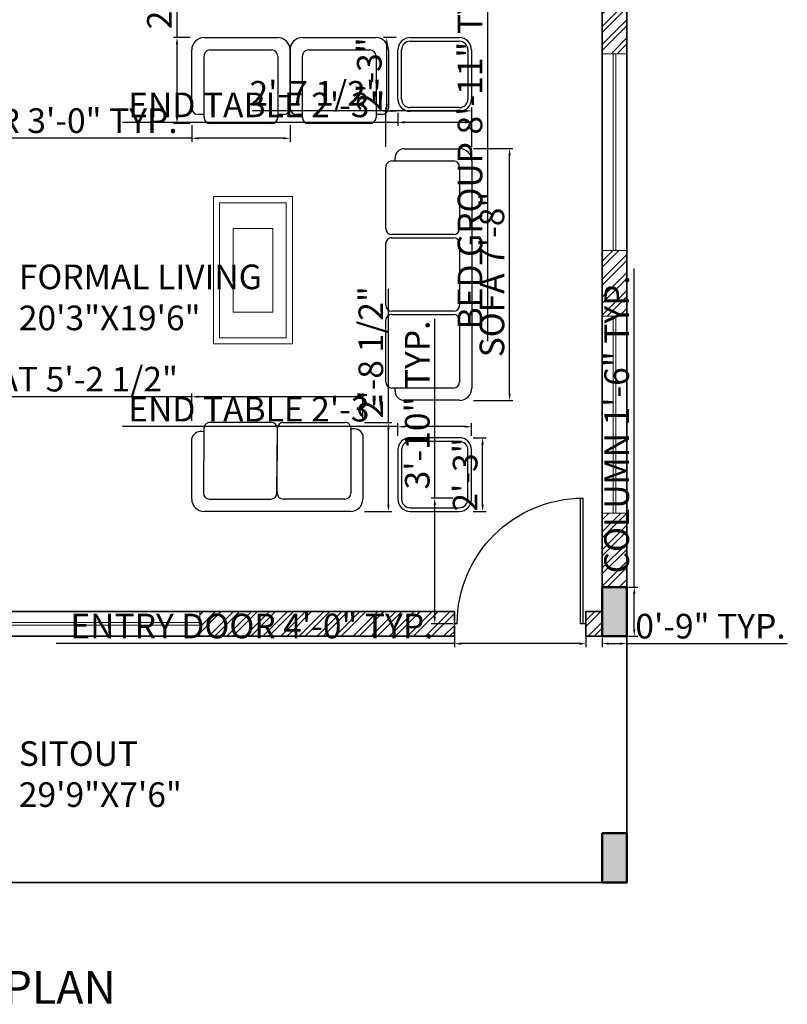
# Model space of a CAD drawing. Units: inches. Extents: x 4153 to 5577, y 785 to 1503.
# Tile 3 of 11: x 4480 to 4761, y 857 to 1217. Entities that reach past the tile are written whole.
import ezdxf

# ---------------------------------------------------------------- set-up
doc = ezdxf.new("R2010")
doc.units = ezdxf.units.IN
for name, color, linetype, lineweight in [('A-ANNO-DIMS', 2, 'Continuous', 18), ('A-ANNO-TEXT', 7, 'Continuous', 35), ('A-AREA-IDEN', 7, 'Continuous', 25), ('A-COLS', 7, 'Continuous', 50), ('A-DOOR', 3, 'Continuous', 25), ('A-FURN', 8, 'Continuous', 18), ('A-GLAZ', 4, 'Continuous', 18), ('A-WALL', 7, 'Continuous', 35)]:
    doc.layers.add(name, color=color, linetype=linetype, lineweight=lineweight)
doc.layers.add('A-WALL-PATT', color=251, linetype='Continuous', lineweight=13, true_color=0x636466)
doc.layers.add('M40-KOLTUKSUNGERI', color=136, linetype='Continuous')
doc.styles.get("Standard").update_dxf_attribs({"font": 'arial.ttf'})
doc.dimstyles.new('ISO-25', dxfattribs={"dimtxt": 9, "dimasz": 2.5, "dimexe": 1.25, "dimexo": 0.625, "dimtad": 1, "dimlunit": 3, "dimtxsty": 'Standard', "dimcen": 2.5, "dimadec": 0, "dimazin": 0, "dimtfac": 1, "dimtmove": 0, "dimatfit": 3, "dimfxl": 1, "dimarcsym": 0})

# ---------------------------------------------------------------- blocks, each defined once
blk = doc.blocks.new('D')
for p, q in [((1, 0), (1, 46)), ((2, 0), (2, 46)), ((0, 0), (2, 0)), ((47, 0), (48, 0))]:
    blk.add_line(p, q)
at = {"ltscale": 0.5}
blk.add_arc((1, 0), 46, 0, 90, dxfattribs=at)
blk = doc.blocks.new('S1')
at = {"layer": 'M40-KOLTUKSUNGERI'}
for p, q in [((3.94, 27.4), (23.53, 27.4)), ((0, -23.47), (0, 23.47)), ((26.59, 23.52), (5.91, 23.65)), ((3.94, 21.68), (3.94, 2.06)), ((28.54, 1.93), (28.54, 21.55)), ((5.91, 0.09), (26.57, -0.04)), ((5.91, 0.03), (26.57, -0.04)), ((3.94, -21.63), (3.94, -1.94)), ((28.54, -1.94), (28.54, -21.67)), ((26.28, -23.6), (5.91, -23.6)), ((24.64, -27.4), (3.94, -27.4))]:
    blk.add_line(p, q, dxfattribs=at)
for centre, radius, start, end in [((3.94, 23.47), 3.94, 90, 180), ((22.44, 24.41), 3.19, 343.8468, 69.9238), ((5.91, 21.68), 1.97, 90, 180), ((26.57, 21.55), 1.97, 360, 90), ((5.91, 2.06), 1.97, 180, 270), ((5.91, -1.94), 1.97, 90, 180), ((26.57, 1.93), 1.97, 270, 0), ((26.57, -2.01), 1.97, 360, 90), ((5.91, -21.63), 1.97, 180, 270), ((26.6, -21.69), 1.94, 260.2828, 0.3826), ((3.94, -23.47), 3.94, 180, 270), ((23.58, -24.69), 2.91, 291.3314, 22.0931)]:
    blk.add_arc(centre, radius, start, end, dxfattribs=at)
blk = doc.blocks.new('S2')
at = {"layer": 'M40-KOLTUKSUNGERI'}
for p, q in [((-36.42, 5.91), (-36.42, 25.59)), ((-34.45, 27.56), (-14.76, 27.56)), ((-12.8, 25.59), (-12.8, 5.91)), ((-11.81, 5.91), (-11.81, 25.59)), ((-9.84, 27.56), (9.84, 27.56)), ((11.81, 25.59), (11.81, 5.91)), ((12.8, 5.91), (12.8, 25.59)), ((14.76, 27.56), (34.45, 27.56)), ((36.42, 25.59), (36.42, 5.91)), ((-37.4, 24.61), (-36.42, 24.61)), ((36.42, 24.61), (37.4, 24.61)), ((-40.35, 3.94), (-40.35, 21.65)), ((40.35, 21.65), (40.35, 3.94)), ((-14.76, 3.94), (-34.45, 3.94)), ((9.84, 3.94), (-9.84, 3.94)), ((34.45, 3.94), (14.76, 3.94)), ((36.42, 0), (-36.42, 0))]:
    blk.add_line(p, q, dxfattribs=at)
for centre, radius, start, end in [((-34.45, 25.59), 1.97, 90, 180), ((-14.76, 25.59), 1.97, 360, 90), ((-9.84, 25.59), 1.97, 90, 180), ((9.84, 25.59), 1.97, 360, 90), ((14.76, 25.59), 1.97, 90, 180), ((34.45, 25.59), 1.97, 360, 90), ((-37.4, 21.65), 2.95, 90, 180), ((37.4, 21.65), 2.95, 360, 90), ((-36.42, 3.94), 3.94, 180, 270), ((-34.45, 5.91), 1.97, 180, 270), ((-14.76, 5.91), 1.97, 270, 0), ((-9.84, 5.91), 1.97, 180, 270), ((9.84, 5.91), 1.97, 270, 0), ((14.76, 5.91), 1.97, 180, 270), ((34.45, 5.91), 1.97, 270, 0), ((36.42, 3.94), 3.94, 270, 0)]:
    blk.add_arc(centre, radius, start, end, dxfattribs=at)
blk = doc.blocks.new('S3')
at = {"layer": 'M40-KOLTUKSUNGERI'}
for p, q in [((-24.61, 11.81), (-24.61, 13.78)), ((-22.64, 15.75), (-3.94, 15.75)), ((-27.56, -9.84), (-27.56, 9.84)), ((-25.59, 11.81), (-5.91, 11.81)), ((-3.94, 9.84), (-3.94, -9.84)), ((0, 11.81), (0, -11.81)), ((-5.91, -11.81), (-25.59, -11.81)), ((-24.61, -13.78), (-24.61, -11.81)), ((-3.94, -15.75), (-22.64, -15.75))]:
    blk.add_line(p, q, dxfattribs=at)
for centre, radius, start, end in [((-22.64, 13.78), 1.97, 90, 180), ((-3.94, 11.81), 3.94, 360, 90), ((-25.59, 9.84), 1.97, 90, 180), ((-5.91, 9.84), 1.97, 360, 90), ((-25.59, -9.84), 1.97, 180, 270), ((-5.91, -9.84), 1.97, 270, 0), ((-3.94, -11.81), 3.94, 270, 0), ((-22.64, -13.78), 1.97, 180, 270)]:
    blk.add_arc(centre, radius, start, end, dxfattribs=at)
blk = doc.blocks.new('T1')
at = {"layer": 'M40-KOLTUKSUNGERI'}
for p, q in [((4762.34, 1687.13), (4746.59, 1687.13)), ((4742.65, 1683.2), (4742.65, 1667.45)), ((4743.83, 1683.2), (4743.83, 1667.45)), ((4762.34, 1685.95), (4746.59, 1685.95)), ((4765.09, 1667.45), (4765.09, 1683.2)), ((4766.27, 1667.45), (4766.27, 1683.2)), ((4746.59, 1664.69), (4762.34, 1664.69)), ((4746.59, 1663.51), (4762.34, 1663.51))]:
    blk.add_line(p, q, dxfattribs=at)
for centre, radius, start, end in [((4746.59, 1683.2), 3.94, 90, 180), ((4762.34, 1683.2), 3.94, 360, 90), ((4746.59, 1683.2), 2.76, 90, 180), ((4762.34, 1683.2), 2.76, 360, 90), ((4746.59, 1667.45), 3.94, 180, 270), ((4746.59, 1667.45), 2.76, 180, 270), ((4762.34, 1667.45), 3.94, 270, 0), ((4762.34, 1667.45), 2.76, 270, 0)]:
    blk.add_arc(centre, radius, start, end, dxfattribs=at)
blk = doc.blocks.new('T2')
at = {"layer": 'M40-KOLTUKSUNGERI'}
for p, q in [((4874.89, 1687.13), (4890.64, 1687.13)), ((4870.95, 1667.45), (4870.95, 1683.2)), ((4872.13, 1667.45), (4872.13, 1683.2)), ((4874.89, 1685.95), (4890.64, 1685.95)), ((4893.39, 1683.2), (4893.39, 1667.45)), ((4894.57, 1683.2), (4894.57, 1667.45)), ((4890.64, 1664.69), (4874.89, 1664.69)), ((4890.64, 1663.51), (4874.89, 1663.51))]:
    blk.add_line(p, q, dxfattribs=at)
for centre, radius, start, end in [((4874.89, 1683.2), 3.94, 90, 180), ((4890.64, 1683.2), 3.94, 360, 90), ((4874.89, 1683.2), 2.76, 90, 180), ((4890.64, 1683.2), 2.76, 360, 90), ((4874.89, 1667.45), 3.94, 180, 270), ((4874.89, 1667.45), 2.76, 180, 270), ((4890.64, 1667.45), 3.94, 270, 0), ((4890.64, 1667.45), 2.76, 270, 0)]:
    blk.add_arc(centre, radius, start, end, dxfattribs=at)
blk = doc.blocks.new('WINDOW-72IN')
for p, q in [((0, 9), (0, 0)), ((72, 9), (72, 0)), ((0, 5), (72, 5)), ((0, 4), (72, 4))]:
    blk.add_line(p, q)
blk = doc.blocks.new('COL-9X18IN')
at = {"transparency": 33554687}
h = blk.add_hatch(color=256, dxfattribs=at)
h.dxf.hatch_style = 1
h.paths.add_polyline_path([(9, 18), (0, 18), (0, 0), (9, 0)])
blk.add_lwpolyline([(0, 18), (9, 18), (9, 0), (0, 0)], close=True)
blk = doc.blocks.new('*D98')
at = {"layer": 'A-ANNO-DIMS', "color": 0, "lineweight": -2, "transparency": 16777216}
for p, q in [((4704.63, 1009.49), (4704.63, 1125.97)), ((4702.55, 1009.49), (4705.88, 1009.49)), ((4704.63, 993.99), (4704.63, 1006.99)), ((4702.55, 991.49), (4705.88, 991.49))]:
    blk.add_line(p, q, dxfattribs=at)
at = {"layer": 'A-ANNO-DIMS', "color": 0, "transparency": 16777216}
for points in [[(4704.21, 1006.99), (4705.04, 1006.99), (4704.63, 1009.49)], [(4704.21, 993.99), (4705.04, 993.99), (4704.63, 991.49)]]:
    blk.add_solid(points, dxfattribs=at)
at = {"layer": 'Defpoints', "color": 0, "transparency": 16777216}
for p in [(4701.93, 1009.49), (4704.63, 1009.49), (4701.93, 991.49)]:
    blk.add_point(p, dxfattribs=at)
at = {"layer": 'A-ANNO-DIMS', "color": 0, "transparency": 16777216, "insert": (4699.35, 1068.98), "char_height": 9, "attachment_point": 5, "rotation": 90}
blk.add_mtext('COLUMN 1\'-6" TYP.', dxfattribs=at)
blk = doc.blocks.new('*D99')
at = {"layer": 'A-ANNO-DIMS', "color": 0, "lineweight": -2, "transparency": 16777216}
for p, q in [((4692.93, 990.86), (4692.93, 987.54)), ((4701.93, 990.86), (4701.93, 987.54)), ((4695.43, 988.79), (4699.43, 988.79)), ((4701.93, 988.79), (4760.54, 988.79))]:
    blk.add_line(p, q, dxfattribs=at)
at = {"layer": 'A-ANNO-DIMS', "color": 0, "transparency": 16777216}
for points in [[(4695.43, 989.21), (4695.43, 988.37), (4692.93, 988.79)], [(4699.43, 989.21), (4699.43, 988.37), (4701.93, 988.79)]]:
    blk.add_solid(points, dxfattribs=at)
at = {"layer": 'Defpoints', "color": 0, "transparency": 16777216}
for p in [(4692.93, 991.49), (4701.93, 991.49), (4701.93, 988.79)]:
    blk.add_point(p, dxfattribs=at)
at = {"layer": 'A-ANNO-DIMS', "color": 0, "transparency": 16777216, "insert": (4732.48, 994.01), "char_height": 9, "attachment_point": 5}
blk.add_mtext('0\'-9" TYP.', dxfattribs=at)
blk = doc.blocks.new('*D112')
at = {"layer": 'A-ANNO-DIMS', "color": 0, "lineweight": -2, "transparency": 16777216}
for p, q in [((4635.6, 1350.66), (4652.3, 1350.66)), ((4651.05, 1348.16), (4651.05, 1245.99)), ((4635.6, 1243.49), (4652.3, 1243.49)), ((4651.05, 1243.49), (4651.05, 1099.34))]:
    blk.add_line(p, q, dxfattribs=at)
at = {"layer": 'A-ANNO-DIMS', "color": 0, "transparency": 16777216}
for points in [[(4650.63, 1348.16), (4651.47, 1348.16), (4651.05, 1350.66)], [(4650.63, 1245.99), (4651.47, 1245.99), (4651.05, 1243.49)]]:
    blk.add_solid(points, dxfattribs=at)
at = {"layer": 'Defpoints', "color": 0, "transparency": 16777216}
for p in [(4634.98, 1350.66), (4634.98, 1243.49), (4651.05, 1243.49)]:
    blk.add_point(p, dxfattribs=at)
at = {"layer": 'A-ANNO-DIMS', "color": 0, "transparency": 16777216, "insert": (4645.77, 1170.17), "char_height": 9, "attachment_point": 5, "rotation": 90}
blk.add_mtext('BED GROUP 8\'-11" TYP.', dxfattribs=at)
blk = doc.blocks.new('*D124')
at = {"layer": 'A-ANNO-DIMS', "color": 0, "lineweight": -2, "transparency": 16777216}
for p, q in [((4542.96, 1070.29), (4542.96, 1080.29)), ((4605.44, 1070.29), (4605.44, 1080.29)), ((4542.96, 1079.04), (4424.83, 1079.04)), ((4602.94, 1079.04), (4545.46, 1079.04))]:
    blk.add_line(p, q, dxfattribs=at)
at = {"layer": 'A-ANNO-DIMS', "color": 0, "transparency": 16777216}
for points in [[(4545.46, 1079.46), (4545.46, 1078.63), (4542.96, 1079.04)], [(4602.94, 1079.46), (4602.94, 1078.63), (4605.44, 1079.04)]]:
    blk.add_solid(points, dxfattribs=at)
at = {"layer": 'Defpoints', "color": 0, "transparency": 16777216}
for p in [(4542.96, 1079.04), (4542.96, 1069.67), (4605.44, 1069.67)]:
    blk.add_point(p, dxfattribs=at)
at = {"layer": 'A-ANNO-DIMS', "color": 0, "transparency": 16777216, "insert": (4482.65, 1084.32), "char_height": 9, "attachment_point": 5}
blk.add_mtext('LOVESEAT 5\'-2 1/2"', dxfattribs=at)
blk = doc.blocks.new('*D125')
at = {"layer": 'A-ANNO-DIMS', "color": 0, "lineweight": -2, "transparency": 16777216}
for p, q in [((4614.81, 1069.67), (4614.81, 1118.47)), ((4606.07, 1069.67), (4616.06, 1069.67)), ((4614.81, 1039.62), (4614.81, 1067.17)), ((4606.07, 1037.12), (4616.06, 1037.12))]:
    blk.add_line(p, q, dxfattribs=at)
at = {"layer": 'A-ANNO-DIMS', "color": 0, "transparency": 16777216}
for points in [[(4614.4, 1067.17), (4615.23, 1067.17), (4614.81, 1069.67)], [(4614.4, 1039.62), (4615.23, 1039.62), (4614.81, 1037.12)]]:
    blk.add_solid(points, dxfattribs=at)
at = {"layer": 'Defpoints', "color": 0, "transparency": 16777216}
for p in [(4605.44, 1069.67), (4614.81, 1069.67), (4605.44, 1037.12)]:
    blk.add_point(p, dxfattribs=at)
at = {"layer": 'A-ANNO-DIMS', "color": 0, "transparency": 16777216, "insert": (4609.54, 1095.32), "char_height": 9, "attachment_point": 5, "rotation": 90}
blk.add_mtext('2\'-8 1/2"', dxfattribs=at)
blk = doc.blocks.new('*D126')
at = {"layer": 'A-ANNO-DIMS', "color": 0, "lineweight": -2, "transparency": 16777216}
for p, q in [((4645.9, 1169.76), (4660.32, 1169.76)), ((4659.07, 1080.24), (4659.07, 1167.26)), ((4645.9, 1077.74), (4660.32, 1077.74))]:
    blk.add_line(p, q, dxfattribs=at)
at = {"layer": 'A-ANNO-DIMS', "color": 0, "transparency": 16777216}
for points in [[(4658.66, 1167.26), (4659.49, 1167.26), (4659.07, 1169.76)], [(4658.66, 1080.24), (4659.49, 1080.24), (4659.07, 1077.74)]]:
    blk.add_solid(points, dxfattribs=at)
at = {"layer": 'Defpoints', "color": 0, "transparency": 16777216}
for p in [(4645.27, 1169.76), (4659.07, 1169.76), (4645.27, 1077.74)]:
    blk.add_point(p, dxfattribs=at)
at = {"layer": 'A-ANNO-DIMS', "color": 0, "transparency": 16777216, "insert": (4653.79, 1123.75), "char_height": 9, "attachment_point": 5, "rotation": 90}
blk.add_mtext('SOFA 7\'-8"', dxfattribs=at)
blk = doc.blocks.new('*D127')
at = {"layer": 'A-ANNO-DIMS', "color": 0, "lineweight": -2, "transparency": 16777216}
for p, q in [((4613.85, 1170.38), (4613.85, 1184.81)), ((4645.27, 1170.38), (4645.27, 1184.81)), ((4613.85, 1183.56), (4565.05, 1183.56)), ((4642.77, 1183.56), (4616.35, 1183.56))]:
    blk.add_line(p, q, dxfattribs=at)
at = {"layer": 'A-ANNO-DIMS', "color": 0, "transparency": 16777216}
for points in [[(4616.35, 1183.98), (4616.35, 1183.14), (4613.85, 1183.56)], [(4642.77, 1183.98), (4642.77, 1183.14), (4645.27, 1183.56)]]:
    blk.add_solid(points, dxfattribs=at)
at = {"layer": 'Defpoints', "color": 0, "transparency": 16777216}
for p in [(4613.85, 1183.56), (4613.85, 1169.76), (4645.27, 1169.76)]:
    blk.add_point(p, dxfattribs=at)
at = {"layer": 'A-ANNO-DIMS', "color": 0, "transparency": 16777216, "insert": (4588.2, 1188.84), "char_height": 9, "attachment_point": 5}
blk.add_mtext('2\'-7 1/2"', dxfattribs=at)
blk = doc.blocks.new('*D128')
at = {"layer": 'A-ANNO-DIMS', "color": 0, "lineweight": -2, "transparency": 16777216}
for p, q in [((4542.96, 1178.31), (4542.96, 1172.3)), ((4578.86, 1178.31), (4578.86, 1172.3)), ((4542.96, 1173.55), (4441.84, 1173.55)), ((4576.36, 1173.55), (4545.46, 1173.55))]:
    blk.add_line(p, q, dxfattribs=at)
at = {"layer": 'A-ANNO-DIMS', "color": 0, "transparency": 16777216}
for points in [[(4545.46, 1173.96), (4545.46, 1173.13), (4542.96, 1173.55)], [(4576.36, 1173.96), (4576.36, 1173.13), (4578.86, 1173.55)]]:
    blk.add_solid(points, dxfattribs=at)
at = {"layer": 'Defpoints', "color": 0, "transparency": 16777216}
for p in [(4542.96, 1178.93), (4578.86, 1178.93), (4542.96, 1173.55)]:
    blk.add_point(p, dxfattribs=at)
at = {"layer": 'A-ANNO-DIMS', "color": 0, "transparency": 16777216, "insert": (4491.15, 1178.83), "char_height": 9, "attachment_point": 5}
blk.add_mtext('CHAIR 3\'-0" TYP.', dxfattribs=at)
blk = doc.blocks.new('*D129')
at = {"layer": 'A-ANNO-DIMS', "color": 0, "lineweight": -2, "transparency": 16777216}
for p, q in [((4537.57, 1210.35), (4537.57, 1290.09)), ((4542.33, 1210.35), (4536.32, 1210.35)), ((4537.57, 1181.43), (4537.57, 1207.85)), ((4542.33, 1178.93), (4536.32, 1178.93))]:
    blk.add_line(p, q, dxfattribs=at)
at = {"layer": 'A-ANNO-DIMS', "color": 0, "transparency": 16777216}
for points in [[(4537.15, 1207.85), (4537.99, 1207.85), (4537.57, 1210.35)], [(4537.15, 1181.43), (4537.99, 1181.43), (4537.57, 1178.93)]]:
    blk.add_solid(points, dxfattribs=at)
at = {"layer": 'Defpoints', "color": 0, "transparency": 16777216}
for p in [(4537.57, 1210.35), (4542.96, 1210.35), (4542.96, 1178.93)]:
    blk.add_point(p, dxfattribs=at)
at = {"layer": 'A-ANNO-DIMS', "color": 0, "transparency": 16777216, "insert": (4532.29, 1251.47), "char_height": 9, "attachment_point": 5, "rotation": 90}
blk.add_mtext('2\'-7 1/2" TYP.', dxfattribs=at)
blk = doc.blocks.new('*D130')
at = {"layer": 'A-ANNO-DIMS', "color": 0, "lineweight": -2, "transparency": 16777216}
for p, q in [((4618.25, 1064.71), (4618.25, 1069.37)), ((4645.19, 1064.71), (4645.19, 1069.37)), ((4618.25, 1068.12), (4517.69, 1068.12)), ((4642.69, 1068.12), (4620.75, 1068.12))]:
    blk.add_line(p, q, dxfattribs=at)
at = {"layer": 'A-ANNO-DIMS', "color": 0, "transparency": 16777216}
for points in [[(4620.75, 1068.54), (4620.75, 1067.7), (4618.25, 1068.12)], [(4642.69, 1068.54), (4642.69, 1067.7), (4645.19, 1068.12)]]:
    blk.add_solid(points, dxfattribs=at)
at = {"layer": 'Defpoints', "color": 0, "transparency": 16777216}
for p in [(4618.25, 1068.12), (4618.25, 1064.08), (4645.19, 1064.08)]:
    blk.add_point(p, dxfattribs=at)
at = {"layer": 'A-ANNO-DIMS', "color": 0, "transparency": 16777216, "insert": (4566.72, 1073.34), "char_height": 9, "attachment_point": 5}
blk.add_mtext('END TABLE 2\'-3"', dxfattribs=at)
blk = doc.blocks.new('*D131')
at = {"layer": 'A-ANNO-DIMS', "color": 0, "lineweight": -2, "transparency": 16777216}
for p, q in [((4645.81, 1064.08), (4650.47, 1064.08)), ((4649.22, 1039.65), (4649.22, 1061.58)), ((4645.81, 1037.15), (4650.47, 1037.15))]:
    blk.add_line(p, q, dxfattribs=at)
at = {"layer": 'A-ANNO-DIMS', "color": 0, "transparency": 16777216}
for points in [[(4648.81, 1061.58), (4649.64, 1061.58), (4649.22, 1064.08)], [(4648.81, 1039.65), (4649.64, 1039.65), (4649.22, 1037.15)]]:
    blk.add_solid(points, dxfattribs=at)
at = {"layer": 'Defpoints', "color": 0, "transparency": 16777216}
for p in [(4645.19, 1064.08), (4649.22, 1064.08), (4645.19, 1037.15)]:
    blk.add_point(p, dxfattribs=at)
at = {"layer": 'A-ANNO-DIMS', "color": 0, "transparency": 16777216, "insert": (4644, 1050.62), "char_height": 9, "attachment_point": 5, "rotation": 90}
blk.add_mtext('2\'-3"', dxfattribs=at)
blk = doc.blocks.new('*D132')
at = {"layer": 'A-ANNO-DIMS', "color": 0, "lineweight": -2, "transparency": 16777216}
for p, q in [((4618.25, 1182.8), (4618.25, 1178.13)), ((4645.19, 1182.8), (4645.19, 1178.13)), ((4618.25, 1179.38), (4517.69, 1179.38)), ((4642.69, 1179.38), (4620.75, 1179.38))]:
    blk.add_line(p, q, dxfattribs=at)
at = {"layer": 'A-ANNO-DIMS', "color": 0, "transparency": 16777216}
for points in [[(4620.75, 1179.8), (4620.75, 1178.96), (4618.25, 1179.38)], [(4642.69, 1179.8), (4642.69, 1178.96), (4645.19, 1179.38)]]:
    blk.add_solid(points, dxfattribs=at)
at = {"layer": 'Defpoints', "color": 0, "transparency": 16777216}
for p in [(4618.25, 1183.42), (4645.19, 1183.42), (4618.25, 1179.38)]:
    blk.add_point(p, dxfattribs=at)
at = {"layer": 'A-ANNO-DIMS', "color": 0, "transparency": 16777216, "insert": (4566.72, 1184.6), "char_height": 9, "attachment_point": 5}
blk.add_mtext('END TABLE 2\'-3"', dxfattribs=at)
blk = doc.blocks.new('*D133')
at = {"layer": 'A-ANNO-DIMS', "color": 0, "lineweight": -2, "transparency": 16777216}
for p, q in [((4617.63, 1210.35), (4612.96, 1210.35)), ((4614.21, 1185.92), (4614.21, 1207.85)), ((4617.63, 1183.42), (4612.96, 1183.42))]:
    blk.add_line(p, q, dxfattribs=at)
at = {"layer": 'A-ANNO-DIMS', "color": 0, "transparency": 16777216}
for points in [[(4613.8, 1207.85), (4614.63, 1207.85), (4614.21, 1210.35)], [(4613.8, 1185.92), (4614.63, 1185.92), (4614.21, 1183.42)]]:
    blk.add_solid(points, dxfattribs=at)
at = {"layer": 'Defpoints', "color": 0, "transparency": 16777216}
for p in [(4614.21, 1210.35), (4618.25, 1210.35), (4618.25, 1183.42)]:
    blk.add_point(p, dxfattribs=at)
at = {"layer": 'A-ANNO-DIMS', "color": 0, "transparency": 16777216, "insert": (4608.99, 1196.89), "char_height": 9, "attachment_point": 5, "rotation": 90}
blk.add_mtext('2\'-3"', dxfattribs=at)
blk = doc.blocks.new('*D144')
at = {"layer": 'A-ANNO-DIMS', "color": 0, "lineweight": -2, "transparency": 16777216}
for p, q in [((4638.93, 995.36), (4638.93, 987.54)), ((4686.93, 995.36), (4686.93, 987.54)), ((4638.93, 988.79), (4493.47, 988.79)), ((4684.43, 988.79), (4641.43, 988.79))]:
    blk.add_line(p, q, dxfattribs=at)
at = {"layer": 'A-ANNO-DIMS', "color": 0, "transparency": 16777216}
for points in [[(4641.43, 989.21), (4641.43, 988.37), (4638.93, 988.79)], [(4684.43, 989.21), (4684.43, 988.37), (4686.93, 988.79)]]:
    blk.add_solid(points, dxfattribs=at)
at = {"layer": 'Defpoints', "color": 0, "transparency": 16777216}
for p in [(4638.93, 995.99), (4686.93, 995.99), (4638.93, 988.79)]:
    blk.add_point(p, dxfattribs=at)
at = {"layer": 'A-ANNO-DIMS', "color": 0, "transparency": 16777216, "insert": (4564.95, 994.07), "char_height": 9, "attachment_point": 5}
blk.add_mtext('ENTRY DOOR 4\'-0" TYP.', dxfattribs=at)
blk = doc.blocks.new('*D145')
at = {"layer": 'A-ANNO-DIMS', "color": 0, "lineweight": -2, "transparency": 16777216}
for p, q in [((4631.73, 1041.99), (4631.73, 1107.58)), ((4638.3, 1041.99), (4630.48, 1041.99)), ((4631.73, 998.49), (4631.73, 1039.49)), ((4638.3, 995.99), (4630.48, 995.99))]:
    blk.add_line(p, q, dxfattribs=at)
at = {"layer": 'A-ANNO-DIMS', "color": 0, "transparency": 16777216}
for points in [[(4631.31, 1039.49), (4632.14, 1039.49), (4631.73, 1041.99)], [(4631.31, 998.49), (4632.14, 998.49), (4631.73, 995.99)]]:
    blk.add_solid(points, dxfattribs=at)
at = {"layer": 'Defpoints', "color": 0, "transparency": 16777216}
for p in [(4631.73, 1041.99), (4638.93, 1041.99), (4638.93, 995.99)]:
    blk.add_point(p, dxfattribs=at)
at = {"layer": 'A-ANNO-DIMS', "color": 0, "transparency": 16777216, "insert": (4626.5, 1076.04), "char_height": 9, "attachment_point": 5, "rotation": 90}
blk.add_mtext('3\'-10" TYP.', dxfattribs=at)

msp = doc.modelspace()

# ---------------------------------------------------------------- hatches: boundary and pattern name
at = {"layer": 'A-WALL-PATT', "transparency": 33554687}
h = msp.add_hatch(dxfattribs=at)
h.set_pattern_fill('ANSI32', color=256, scale=0.49)
h.paths.add_polyline_path([(4344.927, 1138.488), (4281.927, 1138.488), (4281.927, 1234.488), (4296.927, 1234.488), (4296.927, 1243.488), (4269.927, 1243.488), (4269.927, 1234.488), (4275.927, 1234.488), (4275.927, 1138.488), (4203.927, 1138.488), (4203.927, 1168.488), (4194.927, 1168.488), (4194.927, 1088.988), (4203.927, 1088.988), (4203.927, 1129.488), (4338.927, 1129.488), (4338.927, 1105.488), (4344.927, 1105.488)])
h.paths.add_polyline_path([(4203.927, 1040.988), (4194.927, 1040.988), (4194.927, 1009.488), (4203.927, 1009.488)])
h.paths.add_polyline_path([(4278.927, 1000.488), (4203.927, 1000.488), (4203.927, 991.488), (4278.927, 991.488)])
h.paths.add_polyline_path([(4203.927, 991.488), (4194.927, 991.488), (4194.927, 910.488), (4203.927, 910.488)])
h.paths.add_polyline_path([(4335.927, 907.488), (4203.927, 907.488), (4203.927, 901.488), (4335.927, 901.488)])
h.paths.add_polyline_path([(4344.927, 1057.488), (4338.927, 1057.488), (4338.927, 1000.488), (4344.927, 1000.488)])
h.paths.add_polyline_path([(4335.927, 1000.488), (4326.927, 1000.488), (4326.927, 991.488), (4335.927, 991.488)])
h.paths.add_polyline_path([(4368.927, 1000.488), (4344.927, 1000.488), (4344.927, 991.488), (4368.927, 991.488)])
h.paths.add_polyline_path([(4440.927, 1000.488), (4416.927, 1000.488), (4416.927, 991.488), (4440.927, 991.488)])
h.paths.add_polyline_path([(4449.927, 1120.488), (4440.927, 1120.488), (4440.927, 1000.488), (4449.927, 1000.488)])
h.paths.add_polyline_path([(4473.927, 1000.488), (4458.927, 1000.488), (4458.927, 991.488), (4473.927, 991.488)])
h.paths.add_polyline_path([(4638.927, 1000.488), (4545.927, 1000.488), (4545.927, 991.488), (4638.927, 991.488)])
h.paths.add_polyline_path([(4701.927, 1036.488), (4692.927, 1036.488), (4692.927, 1009.488), (4701.927, 1009.488)])
h.paths.add_polyline_path([(4692.927, 1000.488), (4686.927, 1000.488), (4686.927, 991.488), (4692.927, 991.488)])
h.paths.add_polyline_path([(4701.927, 1132.488), (4692.927, 1132.488), (4692.927, 1108.488), (4701.927, 1108.488)])
h.paths.add_polyline_path([(4701.927, 1225.488), (4692.927, 1225.488), (4692.927, 1204.488), (4701.927, 1204.488)])
h.paths.add_polyline_path([(4650.927, 1243.488), (4560.927, 1243.488), (4560.927, 1265.228), (4560.927, 1381.488), (4650.927, 1381.488), (4650.927, 1393.488), (4644.927, 1393.488), (4644.927, 1387.488), (4560.927, 1387.488), (4560.927, 1435.488), (4551.927, 1435.488), (4551.927, 1354.488), (4530.927, 1354.488), (4530.927, 1348.488), (4551.927, 1348.488), (4551.927, 1309.488), (4485.927, 1309.488), (4485.927, 1234.488), (4505.427, 1234.488), (4505.427, 1243.488), (4494.927, 1243.488), (4494.927, 1303.488), (4551.927, 1303.488), (4551.927, 1243.488), (4541.427, 1243.488), (4541.427, 1234.488), (4650.927, 1234.488)])
h.paths.add_polyline_path([(4701.927, 1426.488), (4692.927, 1426.488), (4692.927, 1357.488), (4701.927, 1357.488)])
h.paths.add_polyline_path([(4701.927, 1309.488), (4692.927, 1309.488), (4692.927, 1243.488), (4701.927, 1243.488)])
h.paths.add_polyline_path([(4692.927, 1444.488), (4608.927, 1444.488), (4608.927, 1435.488), (4644.927, 1435.488), (4644.927, 1423.488), (4650.927, 1423.488), (4650.927, 1435.488), (4692.927, 1435.488)])
h.paths.add_polyline_path([(4497.927, 1444.488), (4479.927, 1444.488), (4479.927, 1435.488), (4485.927, 1435.488), (4485.927, 1348.488), (4500.927, 1348.488), (4500.927, 1354.488), (4494.927, 1354.488), (4494.927, 1435.488), (4497.927, 1435.488)])
h.paths.add_polyline_path([(4551.927, 1444.488), (4545.927, 1444.488), (4545.927, 1435.488), (4551.927, 1435.488)])
h.paths.add_polyline_path([(4572.927, 1444.488), (4569.927, 1444.488), (4569.927, 1435.488), (4572.927, 1435.488)])
h.paths.add_polyline_path([(4431.927, 1444.488), (4356.927, 1444.488), (4356.927, 1435.488), (4431.927, 1435.488)])
h.paths.add_polyline_path([(4284.927, 1444.488), (4203.927, 1444.488), (4203.927, 1435.488), (4284.927, 1435.488)])
h.paths.add_polyline_path([(4203.927, 1426.488), (4194.927, 1426.488), (4194.927, 1293.488), (4203.927, 1293.488), (4203.927, 1295.242)])
h.paths.add_polyline_path([(4347.927, 1435.488), (4338.927, 1435.488), (4338.927, 1243.488), (4332.927, 1243.488), (4332.927, 1234.488), (4431.927, 1234.488), (4431.927, 1243.488), (4347.927, 1243.488)])
h.paths.add_polyline_path([(4239.927, 1243.488), (4203.927, 1243.488), (4203.927, 1234.488), (4239.927, 1234.488)], flags=17)
h.paths.add_polyline_path([(4203.927, 1225.488), (4194.927, 1225.488), (4194.927, 1198.488), (4203.927, 1198.488)], flags=17)

# ---------------------------------------------------------------- linework, layer by layer
at = {"layer": 'A-FURN'}
for points in [[(4550.86, 1098.383), (4550.86, 1152.244), (4579.749, 1152.244), (4579.749, 1098.383)], [(4553.104, 1100.627), (4553.104, 1150), (4577.505, 1150), (4577.505, 1100.627)], [(4558.04, 1110.024), (4558.04, 1140.603), (4572.569, 1140.603), (4572.569, 1110.024)]]:
    msp.add_lwpolyline(points, close=True, dxfattribs=at)
at = {"layer": 'A-WALL'}
for p, q in [((4701.927, 1444.488), (4701.927, 901.488)), ((4692.927, 1234.488), (4692.927, 1000.488)), ((4449.927, 1000.488), (4638.927, 1000.488)), ((4638.927, 1000.488), (4638.927, 991.488)), ((4686.927, 1000.488), (4686.927, 991.488)), ((4686.927, 1000.488), (4692.927, 1000.488)), ((4203.927, 991.488), (4638.927, 991.488)), ((4686.927, 991.488), (4701.927, 991.488)), ((4701.927, 901.488), (4194.927, 901.488))]:
    msp.add_line(p, q, dxfattribs=at)

# ---------------------------------------------------------------- block references
at = {"layer": 'A-COLS'}
for p in [(4692.927, 991.488), (4692.927, 901.488)]:
    msp.add_blockref('COL-9X18IN', p, dxfattribs=at)
at = {"layer": 'A-DOOR', "xscale": -1}
msp.add_blockref('D', (4686.927, 995.988), dxfattribs=at)
at = {"layer": 'A-FURN', "xscale": 1.140062553648158, "yscale": 1.140062553648158, "zscale": 1.140062553648158, "rotation": 90}
for name, p in [('S3', (4560.911, 1210.352)), ('S3', (4596.818, 1210.352)), ('T2', (6541.693, -4369.768)), ('S2', (4645.271, 1123.751)), ('S1', (4574.199, 1037.124)), ('T1', (6541.693, -4369.768))]:
    msp.add_blockref(name, p, dxfattribs=at)
at = {"layer": 'A-GLAZ'}
for p, rotation in [((4692.927, 1204.488), 269.9999999999994), ((4692.927, 1108.488), 270.0000000000009)]:
    msp.add_blockref('WINDOW-72IN', p, dxfattribs=dict(at, rotation=rotation))
msp.add_blockref('WINDOW-72IN', (4473.927, 991.488), dxfattribs=at)

# ---------------------------------------------------------------- texts
at = {"layer": 'A-ANNO-TEXT', "insert": (4345.531, 869.133), "char_height": 12, "attachment_point": 1}
msp.add_mtext_dynamic_manual_height_columns('{\\fTimes New Roman|b0|i0|c0|p18;GROUND FLOOR PLAN}', width=197.6934, gutter_width=12.5, heights=[0], dxfattribs=at)
at = {"layer": 'A-AREA-IDEN', "char_height": 9, "attachment_point": 1}
for s, insert in [('{\\fTimes New Roman|b0|i0|c0|p18;FORMAL LIVING\\P20\'3"X19\'6"}', (4479.768, 1127.378)), ('{\\fTimes New Roman|b0|i0|c0|p18;SITOUT\\P29\'9"X7\'6"}', (4479.768, 953.097))]:
    msp.add_mtext_dynamic_manual_height_columns(s, width=119.83324, gutter_width=12.5, heights=[0], dxfattribs=dict(at, insert=insert))

# ---------------------------------------------------------------- dimensions: what is measured, and where the dimension line sits
at = {"layer": 'A-ANNO-DIMS'}
for base, p1, p2, angle, text, picture, middle in [((4651.051, 1243.488), (4634.976, 1350.661), (4634.976, 1243.488), 270, 'BED GROUP <> TYP.', '*D112', (4645.77, 1170.165)), ((4537.571, 1210.352), (4542.957, 1178.933), (4542.957, 1210.352), 90, '<> TYP.', '*D129', (4532.293, 1251.469)), ((4618.254, 1179.382), (4645.185, 1183.421), (4618.254, 1183.421), 180, 'END TABLE <>', '*D132', (4566.722, 1184.605)), ((4542.957, 1173.547), (4578.865, 1178.933), (4542.957, 1178.933), 180, 'CHAIR <> TYP.', '*D128', (4491.149, 1178.828)), ((4659.073, 1169.758), (4645.271, 1077.745), (4645.271, 1169.758), 90, 'SOFA <>', '*D126', (4653.791, 1123.751)), ((4704.627, 1009.488), (4701.927, 991.488), (4701.927, 1009.488), 90, 'COLUMN <> TYP.', '*D98', (4699.346, 1068.98)), ((4542.957, 1079.042), (4605.442, 1069.669), (4542.957, 1069.669), 180, 'LOVESEAT <>', '*D124', (4482.646, 1084.323)), ((4631.727, 1041.988), (4638.927, 995.988), (4638.927, 1041.988), 90, '<> TYP.', '*D145', (4626.504, 1076.036)), ((4618.254, 1068.121), (4645.185, 1064.082), (4618.254, 1064.082), 180, 'END TABLE <>', '*D130', (4566.722, 1073.344)), ((4638.927, 988.788), (4686.927, 995.988), (4638.927, 995.988), 180, 'ENTRY DOOR <> TYP.', '*D144', (4564.951, 994.07))]:
    dim = msp.add_linear_dim(base=base, p1=p1, p2=p2, angle=angle, text=text, dimstyle='ISO-25', override={"dimdec": 1, "dimlfac": 1, "dimrnd": 0, "dimzin": 1, "dimdsep": 46, "dimlunit": 4, "dimfrac": 2}, dxfattribs=at)
    dim.commit()
    dim.dimension.update_dxf_attribs({"geometry": picture, "text_midpoint": middle})
for base, p1, p2, angle, picture, middle in [((4614.215, 1210.352), (4618.254, 1183.421), (4618.254, 1210.352), 90, '*D133', (4608.992, 1196.887)), ((4613.852, 1183.56), (4645.271, 1169.758), (4613.852, 1169.758), 180, '*D127', (4588.202, 1188.838)), ((4614.814, 1069.669), (4605.442, 1037.124), (4605.442, 1069.669), 90, '*D125', (4609.536, 1095.319)), ((4649.225, 1064.082), (4645.185, 1037.151), (4645.185, 1064.082), 90, '*D131', (4644.001, 1050.616))]:
    dim = msp.add_linear_dim(base=base, p1=p1, p2=p2, angle=angle, dimstyle='ISO-25', override={"dimdec": 1, "dimlfac": 1, "dimrnd": 0, "dimzin": 1, "dimdsep": 46, "dimlunit": 4, "dimfrac": 2}, dxfattribs=at)
    dim.commit()
    dim.dimension.update_dxf_attribs({"geometry": picture, "text_midpoint": middle})
dim = msp.add_linear_dim(base=(4701.927, 988.788), p1=(4692.927, 991.488), p2=(4701.927, 991.488), text='<> TYP.', dimstyle='ISO-25', override={"dimdec": 1, "dimlfac": 1, "dimrnd": 0, "dimzin": 1, "dimdsep": 46, "dimlunit": 4, "dimfrac": 2}, dxfattribs=at)
dim.commit()
dim.dimension.update_dxf_attribs({"geometry": '*D99', "text_midpoint": (4732.482, 994.009)})

doc.saveas('drawing.dxf')
